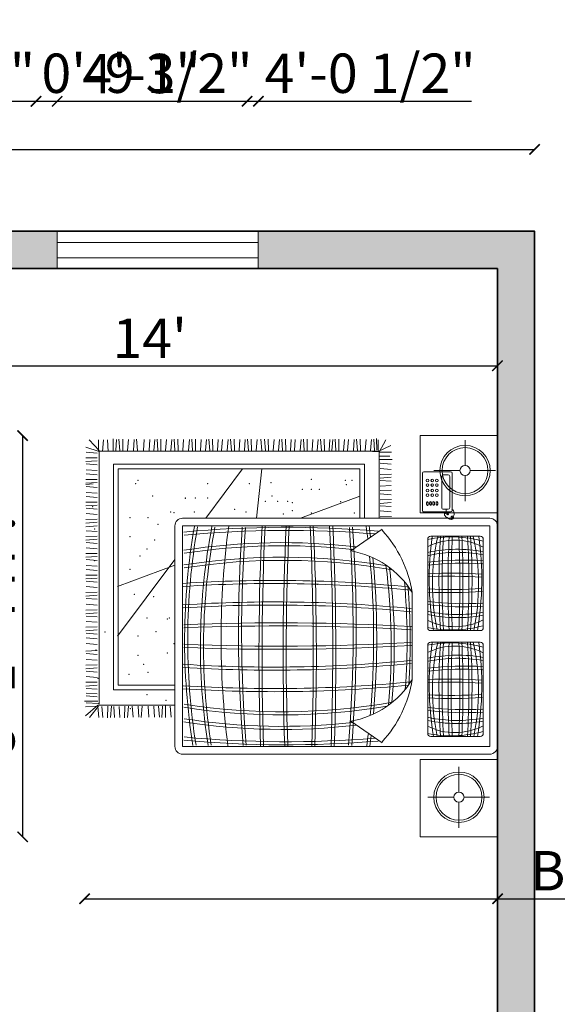
# Model space of a CAD drawing. Units: inches. Extents: x 1704 to 2334, y 1856 to 2559.
# Tile 9 of 10: x 2051 to 2180, y 2321 to 2559. Entities that reach past the tile are written whole.
import ezdxf

# ---------------------------------------------------------------- set-up
doc = ezdxf.new("R2010")
doc.units = ezdxf.units.IN
for name, color, linetype, lineweight in [('A-ANNO-DIMS', 2, 'Continuous', 18), ('A-WALL', 7, 'Continuous', 35), ('BEDS', 17, 'Continuous', 18), ('WINDOW', 6, 'Continuous', 18)]:
    doc.layers.add(name, color=color, linetype=linetype, lineweight=lineweight)
doc.layers.add('A-WALL-PATT', color=18, linetype='Continuous', lineweight=13, true_color=0x000000)
doc.styles.get("Standard").update_dxf_attribs({"font": 'arial.ttf'})
doc.dimstyles.new('ISO-25', dxfattribs={"dimtxt": 9.5, "dimasz": 2.5, "dimexe": 1.25, "dimexo": 0.625, "dimtad": 1, "dimdec": 0, "dimlunit": 4, "dimtxsty": 'Standard', "dimblk": 'ARCHTICK', "dimcen": 2.5, "dimse1": 1, "dimse2": 1, "dimclrd": 3, "dimadec": 0, "dimazin": 0, "dimtfac": 1, "dimtdec": 0, "dimtmove": 0, "dimatfit": 3, "dimfxl": 1, "dimarcsym": 0})

# ---------------------------------------------------------------- blocks, each defined once
blk = doc.blocks.new('A$C77DF40FE')
for p, q in [((0.5, 2.6723), (0, 2.6723)), ((0, 2.6723), (0, 2.1723)), ((0.226, 2.4949), (0.226, 2.6594)), ((0.5, 2.1723), (0.5, 2.6723)), ((0.5339, 0.6344), (0.5339, 2.6214)), ((0.5839, 2.6714), (2.0097, 2.6714)), ((0.5839, 2.6214), (2.0097, 2.6214)), ((0.5839, 0.6344), (0.5839, 2.6214)), ((2.0097, 2.6214), (2.0097, 0.6344)), ((2.0597, 2.6214), (2.0597, 0.6344)), ((2.0936, 2.1723), (2.0936, 2.6723)), ((2.0936, 2.6723), (2.5936, 2.6723)), ((2.3379, 2.4554), (2.3379, 2.6199)), ((2.5936, 2.6723), (2.5936, 2.1723)), ((0.6508, 2.5603), (0.6508, 2.2403)), ((1.2408, 2.5803), (0.6708, 2.5803)), ((1.2608, 2.2403), (1.2608, 2.5603)), ((1.3355, 2.5603), (1.3355, 2.2403)), ((1.9255, 2.5803), (1.3555, 2.5803)), ((1.9455, 2.2403), (1.9455, 2.5603)), ((0.0287, 2.4621), (0.1932, 2.4621)), ((0.226, 2.261), (0.226, 2.4293)), ((0.2588, 2.4621), (0.4233, 2.4621)), ((2.3051, 2.4226), (2.1406, 2.4226)), ((2.5352, 2.4226), (2.3707, 2.4226)), ((0.2338, 2.3688, 10.4), (0.2338, 2.1957, 10.4)), ((0.4828, 2.3788, 10.4), (0.2438, 2.3788, 10.4)), ((0.4656, 2.363, 10.4), (0.2638, 2.363, 10.4)), ((0.4809, 2.3823), (0.4746, 2.3757)), ((0.4873, 2.387), (0.4809, 2.3823)), ((0.4937, 2.3899), (0.4873, 2.387)), ((0.4928, 2.1957, 10.4), (0.4928, 2.3688, 10.4)), ((0.5, 2.3914), (0.4937, 2.3899)), ((0.506, 2.3917), (0.5, 2.3914)), ((0.5117, 2.391), (0.506, 2.3917)), ((0.5168, 2.3897), (0.5117, 2.391)), ((0.5212, 2.3878), (0.5168, 2.3897)), ((0.5205, 2.3816), (0.5202, 2.3804)), ((0.5202, 2.3804), (0.5202, 2.379)), ((0.5202, 2.379), (0.5206, 2.3777)), ((0.521, 2.3828), (0.5205, 2.3816)), ((0.5206, 2.3777), (0.5213, 2.3764)), ((0.5219, 2.3839), (0.521, 2.3828)), ((0.5248, 2.3858), (0.5212, 2.3878)), ((0.5213, 2.3764), (0.5224, 2.3752)), ((0.523, 2.3849), (0.5219, 2.3839)), ((0.5224, 2.3752), (0.5237, 2.374)), ((0.5244, 2.3856), (0.523, 2.3849)), ((0.5237, 2.374), (0.5252, 2.3731)), ((0.5261, 2.3861), (0.5244, 2.3856)), ((0.5277, 2.3836), (0.5248, 2.3858)), ((0.5252, 2.3731), (0.5268, 2.3723)), ((0.5279, 2.3864), (0.5261, 2.3861)), ((0.5268, 2.3723), (0.5283, 2.3719)), ((0.5298, 2.3813), (0.5277, 2.3836)), ((0.5298, 2.3864), (0.5279, 2.3864)), ((0.5283, 2.3719), (0.5297, 2.3717)), ((0.5297, 2.3717), (0.531, 2.372)), ((0.5318, 2.3861), (0.5298, 2.3864)), ((0.5313, 2.3792), (0.5298, 2.3813)), ((0.531, 2.372), (0.5319, 2.3726)), ((0.5322, 2.3771), (0.5313, 2.3792)), ((0.5338, 2.3855), (0.5318, 2.3861)), ((0.5319, 2.3726), (0.5325, 2.3738)), ((0.5326, 2.3753), (0.5322, 2.3771)), ((0.5325, 2.3738), (0.5326, 2.3753)), ((0.5356, 2.3846), (0.5338, 2.3855)), ((0.5373, 2.3832), (0.5356, 2.3846)), ((0.5356, 2.3543), (0.537, 2.3561)), ((0.537, 2.3561), (0.5383, 2.3581)), ((0.5387, 2.3815), (0.5373, 2.3832)), ((0.5383, 2.3581), (0.5394, 2.3604)), ((0.5399, 2.3794), (0.5387, 2.3815)), ((0.5394, 2.3604), (0.5403, 2.3629)), ((0.5407, 2.377), (0.5399, 2.3794)), ((0.5403, 2.3629), (0.5409, 2.3657)), ((0.5412, 2.3743), (0.5407, 2.377)), ((0.5409, 2.3657), (0.5413, 2.3686)), ((0.5414, 2.3715), (0.5412, 2.3743)), ((0.5413, 2.3686), (0.5414, 2.3715)), ((2.3379, 2.2215), (2.3379, 2.3898)), ((0.2538, 2.353, 10.4), (0.2538, 2.3215, 10.4)), ((0.2638, 2.3115, 10.4), (0.4656, 2.3115, 10.4)), ((0.4756, 2.3215, 10.4), (0.4756, 2.353, 10.4)), ((0.4767, 2.3409), (0.4876, 2.34)), ((0.4876, 2.34), (0.4961, 2.3402)), ((0.4961, 2.3402), (0.5023, 2.3413)), ((0.502, 2.3463), (0.5017, 2.3431)), ((0.5017, 2.3431), (0.5018, 2.3398)), ((0.5018, 2.3398), (0.5023, 2.3365)), ((0.5026, 2.3491), (0.502, 2.3463)), ((0.5023, 2.3413), (0.5067, 2.3431)), ((0.5023, 2.3365), (0.5031, 2.3334)), ((0.5035, 2.3514), (0.5026, 2.3491)), ((0.5031, 2.3334), (0.5043, 2.3309)), ((0.5047, 2.3531), (0.5035, 2.3514)), ((0.5043, 2.3309), (0.506, 2.329)), ((0.5059, 2.3542), (0.5047, 2.3531)), ((0.5073, 2.3548), (0.5059, 2.3542)), ((0.506, 2.329), (0.5081, 2.328)), ((0.5067, 2.3431), (0.5095, 2.3452)), ((0.5086, 2.3549), (0.5073, 2.3548)), ((0.5081, 2.328), (0.5106, 2.328)), ((0.5097, 2.3544), (0.5086, 2.3549)), ((0.5095, 2.3452), (0.511, 2.3475)), ((0.5107, 2.3534), (0.5097, 2.3544)), ((0.5106, 2.328), (0.5134, 2.3288)), ((0.5113, 2.3518), (0.5107, 2.3534)), ((0.511, 2.3475), (0.5115, 2.3498)), ((0.5115, 2.3498), (0.5113, 2.3518)), ((0.5134, 2.3288), (0.5163, 2.3304)), ((0.5163, 2.3304), (0.5193, 2.3325)), ((0.5193, 2.3325), (0.5222, 2.3349)), ((0.5222, 2.3349), (0.5249, 2.3374)), ((0.5249, 2.3374), (0.5271, 2.3398)), ((0.5271, 2.3398), (0.5288, 2.3419)), ((0.5288, 2.3419), (0.5299, 2.3436)), ((0.5299, 2.3436), (0.5305, 2.3449)), ((0.53, 2.3482), (0.5302, 2.3488)), ((0.5301, 2.3477), (0.53, 2.3482)), ((0.5303, 2.3472), (0.5301, 2.3477)), ((0.5302, 2.3488), (0.5308, 2.3495)), ((0.5306, 2.3466), (0.5303, 2.3472)), ((0.5305, 2.3449), (0.5307, 2.3459)), ((0.5307, 2.3459), (0.5306, 2.3466)), ((0.5308, 2.3495), (0.5317, 2.3504)), ((0.5317, 2.3504), (0.5329, 2.3515)), ((0.5329, 2.3515), (0.5342, 2.3528)), ((0.5342, 2.3528), (0.5356, 2.3543)), ((0, 2.1723), (0.5, 2.1723)), ((0.2438, 2.1857, 10.4), (0.4828, 2.1857, 10.4)), ((0.6708, 2.2203), (1.2408, 2.2203)), ((1.3555, 2.2203), (1.9255, 2.2203)), ((2.5936, 2.1723), (2.0936, 2.1723)), ((1.5773, 2.1205), (1.0147, 2.1205)), ((0.0644, 1.9807), (0.1019, 1.9003)), ((0.1072, 1.986), (0.1072, 1.911)), ((0.134, 1.9753), (0.134, 1.9057)), ((0.1554, 1.9914), (0.1554, 1.911)), ((0.1792, 1.9138), (0.1849, 1.9847)), ((0.2134, 1.9138), (0.219, 1.9847)), ((0.251, 1.9118), (0.2494, 1.9865)), ((0.2748, 1.9118), (0.2691, 1.9849)), ((0.2899, 1.9138), (0.2956, 1.9847)), ((0.3277, 1.9118), (0.3219, 1.9849)), ((0.3539, 1.9118), (0.3522, 1.9865)), ((0.3766, 1.9138), (0.3822, 1.9847)), ((0.4142, 1.9118), (0.4126, 1.9865)), ((0.438, 1.9118), (0.4323, 1.9849)), ((0.4531, 1.9138), (0.4588, 1.9847)), ((0.4873, 1.9138), (0.493, 1.9847)), ((0.5249, 1.9118), (0.5233, 1.9865)), ((0.1072, 1.9057), (0.0269, 1.9485)), ((0.6051, 1.925), (0.7457, 1.7234)), ((1.9869, 1.925), (1.8463, 1.7234)), ((0.0195, 1.8887), (0.0942, 1.8903)), ((0.0227, 1.8712), (0.0957, 1.8769)), ((0.0247, 1.8561), (0.0955, 1.8504)), ((0.1019, 1.9003), (0.0269, 1.9003)), ((0.1002, 1.8885), (0.1002, 0.0935)), ((0.3112, 1.9057), (0.1019, 1.9057)), ((0.1019, 1.9057), (0.1019, 1.8628)), ((0.5301, 1.9057), (0.3112, 1.9057)), ((0.0227, 1.7843), (0.0974, 1.786)), ((0.0247, 1.8219), (0.0955, 1.8163)), ((0.3112, 1.8116), (0.1852, 1.8116)), ((0.1852, 1.8116), (0.1852, 0.187)), ((0.5339, 1.8116), (0.3112, 1.8116)), ((0.0227, 1.7605), (0.0957, 1.7662)), ((0.0247, 1.7454), (0.0955, 1.7397)), ((0.3112, 1.7816), (0.2152, 1.7816)), ((0.2152, 1.7816), (0.2152, 0.217)), ((0.5339, 1.7816), (0.3112, 1.7816)), ((0.3909, 1.7821), (0.5339, 1.398)), ((0.0247, 1.708), (0.0955, 1.7023)), ((0.0247, 1.6819), (0.0955, 1.6762)), ((0.0227, 1.6443), (0.0974, 1.6459)), ((0.0227, 1.6205), (0.0957, 1.6262)), ((0.0247, 1.6054), (0.0955, 1.5997)), ((0.0227, 1.5505), (0.0974, 1.5521)), ((0.0227, 1.5266), (0.0957, 1.5324)), ((0.0247, 1.5881), (0.0955, 1.5824)), ((0.0247, 1.5116), (0.0955, 1.5059)), ((0.0247, 1.4774), (0.0955, 1.4717)), ((0.0227, 1.4397), (0.0974, 1.4414)), ((0.0227, 1.4159), (0.0957, 1.4217)), ((0.0247, 1.4008), (0.0955, 1.3952)), ((0.0247, 1.3634), (0.0955, 1.3577)), ((0.0247, 1.3374), (0.0955, 1.3317)), ((0.0227, 1.2997), (0.0974, 1.3014)), ((0.0227, 1.2759), (0.0957, 1.2816)), ((0.0247, 1.2608), (0.0955, 1.2551)), ((0.0247, 1.2266), (0.0955, 1.221)), ((0.0227, 1.189), (0.0974, 1.1906)), ((0.0227, 1.1652), (0.0957, 1.1709)), ((0.0227, 1.1414), (0.0957, 1.1471)), ((0.5339, 1.1132), (0.2152, 1.1479)), ((0.0247, 1.1163), (0.0955, 1.1106)), ((0.0227, 1.0786), (0.0974, 1.0803)), ((0.0227, 1.0548), (0.0957, 1.0606)), ((0.0247, 1.0397), (0.0955, 1.0341)), ((0.5339, 0.7837), (0.2152, 1.0221)), ((0.0227, 0.9679), (0.0974, 0.9696)), ((0.0247, 1.0055), (0.0955, 0.9999)), ((0.0227, 0.9441), (0.0957, 0.9498)), ((0.0247, 0.929), (0.0955, 0.9233)), ((0.0247, 0.8916), (0.0955, 0.8859)), ((0.0227, 0.8279), (0.0974, 0.8295)), ((0.0247, 0.8655), (0.0955, 0.8599)), ((0.0227, 0.8041), (0.0957, 0.8098)), ((0.0247, 0.789), (0.0955, 0.7833)), ((0.0227, 0.7172), (0.0974, 0.7188)), ((0.0247, 0.7548), (0.0955, 0.7491)), ((0.0227, 0.6933), (0.0957, 0.6991)), ((0.0247, 0.6783), (0.0955, 0.6726)), ((0.0247, 0.6408), (0.0955, 0.6352)), ((0.0227, 0.6032), (0.0974, 0.6048)), ((0.0227, 0.5794), (0.0957, 0.5851)), ((2.0097, 0.6344), (0.5839, 0.6344)), ((2.0097, 0.5844), (0.5839, 0.5844)), ((1.2963, 0.2134), (0.8003, 0.5844)), ((0.8369, 0.5844), (0.975, 0.2134)), ((1.6139, 0.217), (1.6139, 0.5844)), ((1.6439, 0.187), (1.6439, 0.5844)), ((1.7439, 0.087), (1.7439, 0.5844)), ((0.0247, 0.5643), (0.0955, 0.5586)), ((0.0247, 0.5301), (0.0955, 0.5244)), ((1.8218, 0.5229), (1.7471, 0.5245)), ((1.8197, 0.5605), (1.7489, 0.5548)), ((0.0227, 0.4925), (0.0974, 0.4941)), ((0.0227, 0.4687), (0.0957, 0.4744)), ((0.0247, 0.4536), (0.0955, 0.4479)), ((1.8218, 0.499), (1.7487, 0.5048)), ((1.8197, 0.4839), (1.7489, 0.4783)), ((1.8197, 0.453), (1.7489, 0.4474)), ((0.0247, 0.4227), (0.0955, 0.417)), ((0.0247, 0.3864), (0.0955, 0.3807)), ((1.8197, 0.4168), (1.7489, 0.4111)), ((0.0227, 0.3367), (0.0957, 0.3424)), ((0.0247, 0.3216), (0.0955, 0.3159)), ((1.8218, 0.3671), (1.7487, 0.3728)), ((1.8197, 0.352), (1.7489, 0.3463)), ((0.0247, 0.2842), (0.0955, 0.2785)), ((1.8197, 0.3146), (1.7489, 0.3089)), ((1.7492, 0.2844), (1.8223, 0.2787)), ((1.7492, 0.2606), (1.824, 0.2589)), ((0.0227, 0.2465), (0.0974, 0.2482)), ((0.0227, 0.2227), (0.0957, 0.2285)), ((0.0247, 0.2076), (0.0955, 0.202)), ((0.2152, 0.217), (0.3112, 0.217)), ((0.3112, 0.217), (1.6139, 0.217)), ((1.7513, 0.223), (1.8221, 0.2286)), ((1.7513, 0.1888), (1.8221, 0.1944)), ((0.1019, 0.1857), (0.0216, 0.1857)), ((0.1019, 0.1535), (0.0269, 0.1482)), ((0.1852, 0.187), (0.3112, 0.187)), ((0.3112, 0.187), (1.6439, 0.187)), ((1.7492, 0.1737), (1.8223, 0.1679)), ((1.7492, 0.1499), (1.824, 0.1482)), ((0.1019, 0.116), (0.0269, 0.1214)), ((0.0965, 0.0946), (0.0269, 0.0303)), ((0.1019, 0.0892), (0.0269, 0.0892)), ((0.1019, 0.0946), (0.0751, 0.0089)), ((0.1002, 0.0935), (0.3112, 0.0935)), ((0.107, 0.0096), (0.1126, 0.0804)), ((0.1446, 0.0075), (0.1429, 0.0823)), ((0.1684, 0.0075), (0.1627, 0.0806)), ((0.1835, 0.0096), (0.1892, 0.0804)), ((0.2209, 0.0096), (0.2266, 0.0804)), ((0.247, 0.0096), (0.2527, 0.0804)), ((0.2846, 0.0075), (0.283, 0.0823)), ((0.3084, 0.0075), (0.3027, 0.0806)), ((0.3112, 0.0935), (1.0155, 0.0935)), ((0.3301, 0.0096), (0.3358, 0.0804)), ((0.3676, 0.0096), (0.3732, 0.0804)), ((0.3936, 0.0096), (0.3993, 0.0804)), ((0.4313, 0.0075), (0.4296, 0.0823)), ((0.4551, 0.0075), (0.4493, 0.0806)), ((0.4702, 0.0096), (0.4758, 0.0804)), ((0.5043, 0.0096), (0.51, 0.0804)), ((0.542, 0.0075), (0.5403, 0.0823)), ((0.5658, 0.0075), (0.56, 0.0806)), ((0.5896, 0.0075), (0.5838, 0.0806)), ((0.6147, 0.0096), (0.6204, 0.0804)), ((0.6523, 0.0075), (0.6507, 0.0823)), ((0.6762, 0.0075), (0.6704, 0.0806)), ((0.6912, 0.0096), (0.6969, 0.0804)), ((0.7254, 0.0096), (0.7311, 0.0804)), ((0.7631, 0.0075), (0.7614, 0.0823)), ((0.7869, 0.0075), (0.7811, 0.0806)), ((0.802, 0.0096), (0.8076, 0.0804)), ((0.8394, 0.0096), (0.8451, 0.0804)), ((0.8654, 0.0096), (0.8711, 0.0804)), ((0.9031, 0.0075), (0.9014, 0.0823)), ((0.9269, 0.0075), (0.9212, 0.0806)), ((0.942, 0.0096), (0.9477, 0.0804)), ((0.9762, 0.0096), (0.9818, 0.0804)), ((1.0138, 0.0075), (1.0122, 0.0823)), ((1.0155, 0.0935), (1.7355, 0.0935)), ((1.0376, 0.0075), (1.0319, 0.0806)), ((1.0527, 0.0096), (1.0584, 0.0804)), ((1.0901, 0.0096), (1.0958, 0.0804)), ((1.1278, 0.0075), (1.1261, 0.0823)), ((1.1516, 0.0075), (1.1459, 0.0806)), ((1.1667, 0.0096), (1.1724, 0.0804)), ((1.2009, 0.0096), (1.2065, 0.0804)), ((1.2385, 0.0075), (1.2368, 0.0823)), ((1.2623, 0.0075), (1.2566, 0.0806)), ((1.2774, 0.0096), (1.2831, 0.0804)), ((1.3083, 0.0096), (1.314, 0.0804)), ((1.3446, 0.0096), (1.3503, 0.0804)), ((1.3943, 0.0075), (1.3885, 0.0806)), ((1.4094, 0.0096), (1.415, 0.0804)), ((1.4468, 0.0096), (1.4525, 0.0804)), ((1.4844, 0.0075), (1.4828, 0.0823)), ((1.5083, 0.0075), (1.5025, 0.0806)), ((1.5233, 0.0096), (1.529, 0.0804)), ((1.5575, 0.0096), (1.5632, 0.0804)), ((1.5951, 0.0075), (1.5935, 0.0823)), ((1.619, 0.0075), (1.6132, 0.0806)), ((1.6341, 0.0096), (1.6397, 0.0804)), ((1.665, 0.0096), (1.6706, 0.0804)), ((1.6831, 0.0096), (1.6888, 0.0804)), ((1.7162, 0.0857), (1.7162, 0)), ((1.7323, 0.0911), (1.7269, 0.0107)), ((1.743, 0.0857), (1.8126, 0.0054)), ((1.7483, 0.0911), (1.8233, 0.0322)), ((1.7483, 0.0857), (1.7537, 0.0054)), ((1.7513, 0.1122), (1.8221, 0.1179)), ((1.7513, 0.0858), (1.8221, 0.0915)), ((0.3151, 0.0075), (0.3112, 0.0565))]:
    blk.add_line(p, q)
for centre, radius in [((0.226, 2.4621), 0.1629), ((0.226, 2.4621), 0.1484), ((2.3379, 2.4226), 0.1629), ((2.3379, 2.4226), 0.1484), ((0.226, 2.4621), 0.0328), ((2.3379, 2.4226), 0.0328), ((0.2896, 2.2801, 10.4), 0.00858), ((0.2896, 2.25, 10.4), 0.00858), ((0.3196, 2.2801, 10.4), 0.00858), ((0.3196, 2.25, 10.4), 0.00858), ((0.3554, 2.2801, 10.4), 0.00858), ((0.3554, 2.25, 10.4), 0.00858), ((0.3855, 2.2801, 10.4), 0.00858), ((0.3855, 2.25, 10.4), 0.00858), ((0.2896, 2.2186, 10.4), 0.00858), ((0.3196, 2.2186, 10.4), 0.00858), ((0.3554, 2.2186, 10.4), 0.00858), ((0.3855, 2.2186, 10.4), 0.00858)]:
    blk.add_circle(centre, radius)
for centre, radius, start, end in [((0.5839, 2.6214), 0.05, 90, 180), ((2.0097, 2.6214), 0.05, 0, 90), ((0.6708, 2.5603), 0.02, 90, 180), ((0.9635, 1.1066), 1.4427, 78.1527, 102.49062), ((0.9287, 0.5819), 1.9884, 80.42006, 97.96719), ((1.4247, 2.3742), 0.7696, 164.61122, 191.56793), ((1.0701, 2.3966), 0.3942, 152.53654, 206.92003), ((1.6628, 2.4129), 0.928, 169.60866, 191.89899), ((1.6628, 2.4129), 0.908, 169.60866, 191.89899), ((2.7571, 2.4533), 1.9523, 176.39469, 186.81952), ((2.7571, 2.4533), 1.9323, 176.39469, 186.81952), ((3.9259, 2.3685), 3.0367, 176.14325, 182.77497), ((3.9259, 2.3685), 3.0167, 176.14325, 182.77497), ((-2.0216, 2.3685), 3.0167, 357.22503, 3.85675), ((-2.0216, 2.3685), 3.0367, 357.22503, 3.85675), ((-0.8455, 2.4533), 1.9323, 353.18048, 3.60531), ((-0.8455, 2.4533), 1.9523, 353.18048, 3.60531), ((0.2489, 2.4129), 0.908, 348.10101, 10.39134), ((0.2489, 2.4129), 0.928, 348.10101, 10.39134), ((0.8416, 2.3966), 0.3942, 333.07997, 27.46346), ((0.4869, 2.3742), 0.7696, 348.43207, 15.38878), ((1.2408, 2.5603), 0.02, 0, 90), ((1.3555, 2.5603), 0.02, 90, 180), ((1.6482, 1.1066), 1.4427, 78.1527, 102.49062), ((1.6135, 0.5819), 1.9884, 80.42006, 97.96719), ((2.1094, 2.3742), 0.7696, 164.61122, 191.56793), ((1.7548, 2.3966), 0.3942, 152.53654, 206.92003), ((2.3475, 2.4129), 0.928, 169.60866, 191.89899), ((2.3475, 2.4129), 0.908, 169.60866, 191.89899), ((3.4419, 2.4533), 1.9523, 176.39469, 186.81952), ((3.4419, 2.4533), 1.9323, 176.39469, 186.81952), ((4.6106, 2.3685), 3.0367, 176.14325, 182.77497), ((4.6106, 2.3685), 3.0167, 176.14325, 182.77497), ((-1.3369, 2.3685), 3.0167, 357.22503, 3.85675), ((-1.3369, 2.3685), 3.0367, 357.22503, 3.85675), ((-0.1608, 2.4533), 1.9323, 353.18048, 3.60531), ((-0.1608, 2.4533), 1.9523, 353.18048, 3.60531), ((0.9336, 2.4129), 0.908, 348.10101, 10.39134), ((0.9336, 2.4129), 0.928, 348.10101, 10.39134), ((1.5263, 2.3966), 0.3942, 333.07997, 27.46346), ((1.1716, 2.3742), 0.7696, 348.43207, 15.38878), ((1.9255, 2.5603), 0.02, 0, 90), ((0.9445, -2.3575), 4.8647, 86.26705, 93.45634), ((0.9445, -2.3575), 4.8447, 86.26705, 93.45634), ((1.6292, -2.3575), 4.8647, 86.26705, 93.45634), ((1.6292, -2.3575), 4.8447, 86.26705, 93.45634), ((0.9561, -3.928), 6.3765, 87.24779, 92.75221), ((0.9561, -3.928), 6.3565, 87.24779, 92.75221), ((1.6408, -3.928), 6.3765, 87.24779, 92.75221), ((1.6408, -3.928), 6.3565, 87.24779, 92.75221), ((0.2438, 2.3688, 10.4), 0.01, 90, 180), ((0.2638, 2.353, 10.4), 0.01, 90, 180), ((0.4656, 2.353, 10.4), 0.01, 0, 90), ((0.4828, 2.3688, 10.4), 0.01, 0, 90), ((0.9561, 8.7285), 6.3765, 267.24779, 272.75221), ((0.9561, 8.7285), 6.3565, 267.24779, 272.75221), ((1.6408, 8.7285), 6.3765, 267.24779, 272.75221), ((1.6408, 8.7285), 6.3565, 267.24779, 272.75221), ((0.2638, 2.3215, 10.4), 0.01, 180, 270), ((0.4656, 2.3215, 10.4), 0.01, 270, 0), ((0.9445, 7.158), 4.8647, 266.54366, 273.73295), ((0.9445, 7.158), 4.8447, 266.54366, 273.73295), ((1.6292, 7.158), 4.8647, 266.54366, 273.73295), ((1.6292, 7.158), 4.8447, 266.54366, 273.73295), ((0.43, 2.2801, 10.4), 0.00304, 140.36073, 180), ((0.43, 2.2801, 10.4), 0.00304, 180, 219.63927), ((0.43, 2.2586, 10.4), 0.00304, 140.36073, 180), ((0.43, 2.2586, 10.4), 0.00304, 180, 219.63927), ((0.43, 2.2386, 10.4), 0.00304, 140.36073, 180), ((0.43, 2.2386, 10.4), 0.00304, 180, 219.63927), ((0.434, 2.2768, 10.4), 0.00822, 116.56505, 140.36073), ((0.434, 2.2834, 10.4), 0.00822, 219.63927, 243.43495), ((0.434, 2.2553, 10.4), 0.00822, 116.56505, 140.36073), ((0.434, 2.2619, 10.4), 0.00822, 219.63927, 243.43495), ((0.434, 2.2353, 10.4), 0.00822, 116.56505, 140.36073), ((0.434, 2.2419, 10.4), 0.00822, 219.63927, 243.43495), ((0.4367, 2.2714, 10.4), 0.0142, 101.70092, 116.56505), ((0.4367, 2.2887, 10.4), 0.0142, 243.43495, 258.29908), ((0.4367, 2.25, 10.4), 0.0142, 101.70092, 116.56505), ((0.4367, 2.2673, 10.4), 0.0142, 243.43495, 258.29908), ((0.4367, 2.23, 10.4), 0.0142, 101.70092, 116.56505), ((0.4367, 2.2472, 10.4), 0.0142, 243.43495, 258.29908), ((0.4384, 2.263, 10.4), 0.0228, 90, 101.70092), ((0.4384, 2.2972, 10.4), 0.0228, 258.29908, 270), ((0.4384, 2.2415, 10.4), 0.0228, 90, 101.70092), ((0.4384, 2.2757, 10.4), 0.0228, 258.29908, 270), ((0.4384, 2.2215, 10.4), 0.0228, 90, 101.70092), ((0.4384, 2.2557, 10.4), 0.0228, 258.29908, 270), ((0.4384, 2.263, 10.4), 0.0228, 78.29908, 90), ((0.4384, 2.2972, 10.4), 0.0228, 270, 281.70092), ((0.4384, 2.2415, 10.4), 0.0228, 78.29908, 90), ((0.4384, 2.2757, 10.4), 0.0228, 270, 281.70092), ((0.4384, 2.2215, 10.4), 0.0228, 78.29908, 90), ((0.4384, 2.2557, 10.4), 0.0228, 270, 281.70092), ((0.4402, 2.2714, 10.4), 0.0142, 63.43495, 78.29908), ((0.4402, 2.2887, 10.4), 0.0142, 281.70092, 296.56505), ((0.4402, 2.25, 10.4), 0.0142, 63.43495, 78.29908), ((0.4402, 2.2673, 10.4), 0.0142, 281.70092, 296.56505), ((0.4402, 2.23, 10.4), 0.0142, 63.43495, 78.29908), ((0.4402, 2.2472, 10.4), 0.0142, 281.70092, 296.56505), ((0.4428, 2.2768, 10.4), 0.00822, 39.63927, 63.43495), ((0.4428, 2.2834, 10.4), 0.00822, 296.56505, 320.36073), ((0.4428, 2.2553, 10.4), 0.00822, 39.63927, 63.43495), ((0.4428, 2.2619, 10.4), 0.00822, 296.56505, 320.36073), ((0.4428, 2.2353, 10.4), 0.00822, 39.63927, 63.43495), ((0.4428, 2.2419, 10.4), 0.00822, 296.56505, 320.36073), ((0.4468, 2.2801, 10.4), 0.00304, 0, 39.63927), ((0.4468, 2.2801, 10.4), 0.00304, 320.36073, 0), ((0.4468, 2.2586, 10.4), 0.00304, 0, 39.63927), ((0.4468, 2.2586, 10.4), 0.00304, 320.36073, 0), ((0.4468, 2.2386, 10.4), 0.00304, 0, 39.63927), ((0.4468, 2.2386, 10.4), 0.00304, 320.36073, 0), ((0.6708, 2.2403), 0.02, 180, 270), ((0.9635, 3.6939), 1.4427, 257.50938, 281.8473), ((0.9287, 4.2186), 1.9884, 262.03281, 279.57994), ((1.2408, 2.2403), 0.02, 270, 0), ((1.3555, 2.2403), 0.02, 180, 270), ((1.6482, 3.6939), 1.4427, 257.50938, 281.8473), ((1.6135, 4.2186), 1.9884, 262.03281, 279.57994), ((1.9255, 2.2403), 0.02, 270, 0), ((0.2438, 2.1957, 10.4), 0.01, 180, 270), ((0.4314, 2.2186, 10.4), 0.00304, 140.36073, 180), ((0.4314, 2.2186, 10.4), 0.00304, 180, 219.63927), ((0.4354, 2.2153, 10.4), 0.00822, 116.56505, 140.36073), ((0.4354, 2.2219, 10.4), 0.00822, 219.63927, 243.43495), ((0.4381, 2.2099, 10.4), 0.0142, 101.70092, 116.56505), ((0.4381, 2.2272, 10.4), 0.0142, 243.43495, 258.29908), ((0.4398, 2.2015, 10.4), 0.0228, 90, 101.70092), ((0.4398, 2.2357, 10.4), 0.0228, 258.29908, 270), ((0.4398, 2.2015, 10.4), 0.0228, 78.29908, 90), ((0.4398, 2.2357, 10.4), 0.0228, 270, 281.70092), ((0.4416, 2.2099, 10.4), 0.0142, 63.43495, 78.29908), ((0.4416, 2.2272, 10.4), 0.0142, 281.70092, 296.56505), ((0.4443, 2.2153, 10.4), 0.00822, 39.63927, 63.43495), ((0.4443, 2.2219, 10.4), 0.00822, 296.56505, 320.36073), ((0.4483, 2.2186, 10.4), 0.00304, 0, 39.63927), ((0.4483, 2.2186, 10.4), 0.00304, 320.36073, 0), ((0.4828, 2.1957, 10.4), 0.01, 270, 0), ((1.1396, 1.3485), 0.782, 99.19081, 132.51156), ((1.3217, 1.6229), 0.5847, 121.66764, 170.10648), ((10.1174, 1.2237), 9.161, 174.43278, 183.67204), ((1.3248, -2.1722), 4.2793, 86.15317, 94.70908), ((10.2564, 1.2237), 9.181, 174.43278, 183.67204), ((10.2564, 1.2237), 9.161, 174.43278, 183.67204), ((16.3019, 1.253), 15.0916, 176.72768, 182.32074), ((16.3019, 1.253), 15.0716, 176.72768, 182.32074), ((-13.7099, 1.253), 15.0716, 357.67926, 3.27232), ((-13.7099, 1.253), 15.0916, 357.67926, 3.27232), ((-7.6644, 1.2237), 9.161, 356.32796, 5.56722), ((-7.6644, 1.2237), 9.181, 356.32796, 5.56722), ((1.2703, 1.6229), 0.5847, 9.89352, 58.33236), ((1.4523, 1.3485), 0.782, 47.48844, 80.80919), ((-7.5254, 1.2237), 9.161, 356.32796, 5.55658), ((10.1174, 1.2237), 9.181, 174.54912, 183.67204), ((1.3248, -2.1722), 4.2593, 85.74731, 95.1159), ((-7.5254, 1.2237), 9.181, 356.32796, 5.45088), ((4.947, 1.2796), 4.1406, 170.09388, 188.81788), ((1.3657, -2.1044), 4.0888, 84.7053, 97.42828), ((1.3657, -2.1044), 4.1088, 84.96186, 97.17068), ((-2.355, 1.2796), 4.1406, 351.18212, 9.90612), ((4.947, 1.2796), 4.1606, 170.62723, 188.81788), ((-2.355, 1.2796), 4.1606, 351.18212, 9.37277), ((1.3142, -3.5764), 5.4671, 96.90782, 97.69237), ((7.8077, 1.3061), 7.2149, 175.27403, 185.28261), ((7.8077, 1.3061), 7.1949, 175.41729, 185.28261), ((1.3142, -3.5764), 5.4471, 84.77918, 95.62141), ((1.3142, -3.5764), 5.4671, 84.89528, 95.50522), ((1.3142, -3.5764), 5.4671, 82.70251, 83.44735), ((-5.2157, 1.3061), 7.1949, 354.71739, 4.58271), ((-5.2157, 1.3061), 7.2149, 354.71739, 4.72597), ((1.3142, -3.5764), 5.4471, 96.79597, 97.69237), ((1.3142, -3.5764), 5.4471, 82.70251, 83.56088), ((1.2659, -7.4764), 9.2344, 85.41732, 94.18368), ((1.2659, -7.4764), 9.2144, 85.41732, 94.18368), ((4.8527, 1.2796), 4.1606, 173.36767, 188.81788), ((4.8527, 1.2796), 4.1406, 173.68117, 188.81788), ((-2.2608, 1.2796), 4.1406, 351.18212, 6.31883), ((-2.2608, 1.2796), 4.1606, 351.18212, 6.63233), ((1.4138, -15.5462), 17.172, 88.01473, 92.775), ((1.4138, -15.5462), 17.152, 88.01473, 92.775), ((1.4138, -15.6721), 17.172, 88.01473, 92.775), ((1.4138, -15.6721), 17.152, 88.01473, 92.775), ((1.4138, 18.4566), 17.172, 267.225, 271.98527), ((1.4138, 18.4566), 17.152, 267.225, 271.98527), ((1.4138, 18.3004), 17.172, 267.225, 271.98527), ((1.4138, 18.3004), 17.152, 267.225, 271.98527), ((1.2659, 10.2305), 9.2344, 265.81632, 274.58268), ((1.2659, 10.2305), 9.2144, 265.81632, 274.58268), ((1.3142, 6.3306), 5.4471, 262.30763, 277.29749), ((1.3657, 4.8586), 4.0888, 259.07937, 278.93274), ((1.3657, 4.8586), 4.1088, 259.07937, 278.93274), ((1.3248, 4.9264), 4.2793, 260.07608, 279.1287), ((1.3248, 4.9264), 4.2593, 260.07608, 279.1287), ((0.5839, 0.6344), 0.05, 180, 270), ((2.0097, 0.6344), 0.05, 270, 0)]:
    blk.add_arc(centre, radius, start, end)
for p in [(0.2895, 1.7311), (0.5004, 1.7457), (0.2895, 1.6873), (0.3179, 1.6946), (0.4274, 1.6581), (0.2822, 1.4684), (0.3471, 1.5195), (0.3471, 1.4684), (0.5004, 1.4684), (0.9622, 1.5058), (0.3471, 1.41), (0.4326, 1.3443), (0.4858, 1.3444), (0.4253, 1.3151), (0.5077, 1.286), (0.3909, 1.213), (0.4253, 1.2495), (0.3041, 1.2057), (0.4253, 1.1692), (0.3106, 1.0671), (0.4931, 1.0452), (0.4765, 0.9722), (0.3114, 0.7971), (0.4034, 0.7971), (0.4034, 0.7169), (0.4931, 0.7096), (0.4034, 0.6512), (0.4055, 0.6512), (0.4984, 0.5782), (1.3453, 0.5782), (0.4931, 0.5564), (1.1794, 0.5491), (1.1867, 0.5345), (1.4058, 0.5345), (1.7124, 0.5272), (0.5734, 0.4761), (0.6757, 0.4542), (1.0407, 0.4469), (1.2671, 0.4615), (0.3909, 0.4396), (0.5296, 0.4104), (0.7341, 0.4032), (1.1794, 0.4032), (1.5299, 0.4104), (1.6759, 0.4032), (0.2895, 0.3448), (0.3114, 0.3302), (0.7779, 0.3594), (1.0261, 0.3229), (1.2963, 0.3448), (1.4204, 0.3448), (1.4788, 0.3813), (0.5296, 0.2937), (0.6538, 0.2937), (0.8655, 0.2937), (1.5445, 0.2864), (1.7652, 0.2958), (1.2693, 0.1315), (0.6049, 0.0659), (0.8093, 0.0659), (1.3861, 0.0732), (1.5686, 0.0878), (0.4588, 0.0513)]:
    blk.add_point(p)
blk = doc.blocks.new('_ArchTick')
at = {"color": 0, "linetype": 'ByBlock', "const_width": 0.15}
blk.add_lwpolyline([(-0.5, -0.5), (0.5, 0.5)], dxfattribs=at)
blk = doc.blocks.new('*D14')
at = {"layer": 'A-ANNO-DIMS', "color": 0, "lineweight": -2, "transparency": 16777216}
blk.add_line((1998.01, 2475.56), (2166.01, 2475.56), dxfattribs=at)
at = {"layer": 'Defpoints', "color": 0, "transparency": 16777216}
for p in [(2166.01, 2475.56), (1998.01, 2469.33), (2166.01, 2469.33)]:
    blk.add_point(p, dxfattribs=at)
at = {"layer": 'A-ANNO-DIMS', "color": 0, "lineweight": -2, "transparency": 16777216, "xscale": 2.5, "yscale": 2.5, "zscale": 2.5, "rotation": 180}
blk.add_blockref('_ArchTick', (1998.01, 2475.56), dxfattribs=at)
at = {"layer": 'A-ANNO-DIMS', "color": 0, "lineweight": -2, "transparency": 16777216, "xscale": 2.5, "yscale": 2.5, "zscale": 2.5}
blk.add_blockref('_ArchTick', (2166.01, 2475.56), dxfattribs=at)
at = {"layer": 'A-ANNO-DIMS', "color": 0, "transparency": 16777216, "insert": (2082.01, 2480.96), "char_height": 9.5, "attachment_point": 5}
blk.add_mtext("14'", dxfattribs=at)
blk = doc.blocks.new('*D22')
at = {"layer": 'A-ANNO-DIMS', "color": 0, "lineweight": -2, "transparency": 16777216}
blk.add_line((1755.01, 2527.77), (2175.01, 2527.77), dxfattribs=at)
at = {"layer": 'Defpoints', "color": 0, "transparency": 16777216}
for p in [(2175.01, 2527.77), (1755.01, 2508.04), (2175.01, 2508.04)]:
    blk.add_point(p, dxfattribs=at)
at = {"layer": 'A-ANNO-DIMS', "color": 0, "lineweight": -2, "transparency": 16777216, "xscale": 2.5, "yscale": 2.5, "zscale": 2.5, "rotation": 180}
blk.add_blockref('_ArchTick', (1755.01, 2527.77), dxfattribs=at)
at = {"layer": 'A-ANNO-DIMS', "color": 0, "lineweight": -2, "transparency": 16777216, "xscale": 2.5, "yscale": 2.5, "zscale": 2.5}
blk.add_blockref('_ArchTick', (2175.01, 2527.77), dxfattribs=at)
at = {"layer": 'A-ANNO-DIMS', "color": 0, "transparency": 16777216, "insert": (1965.01, 2533.25), "char_height": 9.5, "attachment_point": 5}
blk.add_mtext("35'", dxfattribs=at)
blk = doc.blocks.new('*D24')
at = {"layer": 'A-ANNO-DIMS', "color": 3, "lineweight": -2, "transparency": 16777216}
for p, q in [((2066.27, 2346.88), (2166.04, 2346.88)), ((2166.04, 2346.88), (2334.22, 2346.88))]:
    blk.add_line(p, q, dxfattribs=at)
at = {"layer": 'Defpoints', "color": 0, "transparency": 16777216}
for p in [(2066.27, 2361.85), (2166.04, 2361.85), (2166.04, 2346.88)]:
    blk.add_point(p, dxfattribs=at)
at = {"layer": 'A-ANNO-DIMS', "color": 3, "lineweight": -2, "transparency": 16777216, "xscale": 2.5, "yscale": 2.5, "zscale": 2.5, "rotation": 180}
blk.add_blockref('_ArchTick', (2066.27, 2346.88), dxfattribs=at)
at = {"layer": 'A-ANNO-DIMS', "color": 3, "lineweight": -2, "transparency": 16777216, "xscale": 2.5, "yscale": 2.5, "zscale": 2.5}
blk.add_blockref('_ArchTick', (2166.04, 2346.88), dxfattribs=at)
at = {"layer": 'A-ANNO-DIMS', "color": 0, "transparency": 16777216, "insert": (2251.38, 2352.42), "char_height": 9.5, "attachment_point": 5}
blk.add_mtext('BED ENSEMBLE 8\'-4" TYP.', dxfattribs=at)
blk = doc.blocks.new('*D25')
at = {"layer": 'A-ANNO-DIMS', "color": 3, "lineweight": -2, "transparency": 16777216}
blk.add_line((2051.3, 2458.69), (2051.3, 2361.85), dxfattribs=at)
at = {"layer": 'Defpoints', "color": 0, "transparency": 16777216}
for p in [(2066.27, 2458.69), (2051.3, 2361.85), (2066.27, 2361.85)]:
    blk.add_point(p, dxfattribs=at)
at = {"layer": 'A-ANNO-DIMS', "color": 3, "lineweight": -2, "transparency": 16777216, "xscale": 2.5, "yscale": 2.5, "zscale": 2.5}
for p, rotation in [((2051.3, 2458.69), 90), ((2051.3, 2361.85), 270)]:
    blk.add_blockref('_ArchTick', p, dxfattribs=dict(at, rotation=rotation))
at = {"layer": 'A-ANNO-DIMS', "color": 0, "transparency": 16777216, "insert": (2045.83, 2410.27), "char_height": 9.5, "attachment_point": 5, "rotation": 90}
blk.add_mtext('8\'-1" TYP.', dxfattribs=at)
blk = doc.blocks.new('*D36')
at = {"layer": 'A-ANNO-DIMS', "color": 3, "lineweight": -2, "transparency": 16777216}
blk.add_line((2206.36, 2319.04), (2206.36, 2499.04), dxfattribs=at)
at = {"layer": 'Defpoints', "color": 0, "transparency": 16777216}
for p in [(2166.01, 2499.04), (2206.36, 2499.04), (2166.01, 2319.04)]:
    blk.add_point(p, dxfattribs=at)
at = {"layer": 'A-ANNO-DIMS', "color": 3, "lineweight": -2, "transparency": 16777216, "xscale": 2.5, "yscale": 2.5, "zscale": 2.5}
for p, rotation in [((2206.36, 2499.04), 90), ((2206.36, 2319.04), 270)]:
    blk.add_blockref('_ArchTick', p, dxfattribs=dict(at, rotation=rotation))
at = {"layer": 'A-ANNO-DIMS', "color": 0, "transparency": 16777216, "insert": (2200.88, 2409.04), "char_height": 9.5, "attachment_point": 5, "rotation": 90}
blk.add_mtext('15\'-0"', dxfattribs=at)
blk = doc.blocks.new('*D51')
at = {"layer": 'A-ANNO-DIMS', "color": 3, "lineweight": -2, "transparency": 16777216}
for p, q in [((2045.28, 2539.39), (2054.53, 2539.39)), ((2054.53, 2539.39), (2105.67, 2539.39))]:
    blk.add_line(p, q, dxfattribs=at)
at = {"layer": 'Defpoints', "color": 0, "transparency": 16777216}
for p in [(2054.53, 2539.39), (2045.28, 2117.04), (2054.53, 2117.04)]:
    blk.add_point(p, dxfattribs=at)
at = {"layer": 'A-ANNO-DIMS', "color": 3, "lineweight": -2, "transparency": 16777216, "xscale": 2.5, "yscale": 2.5, "zscale": 2.5, "rotation": 180}
blk.add_blockref('_ArchTick', (2045.28, 2539.39), dxfattribs=at)
at = {"layer": 'A-ANNO-DIMS', "color": 3, "lineweight": -2, "transparency": 16777216, "xscale": 2.5, "yscale": 2.5, "zscale": 2.5}
blk.add_blockref('_ArchTick', (2054.53, 2539.39), dxfattribs=at)
at = {"layer": 'A-ANNO-DIMS', "color": 0, "transparency": 16777216, "insert": (2081.35, 2544.93), "char_height": 9.5, "attachment_point": 5}
blk.add_mtext('0\'-9 1/2"', dxfattribs=at)
blk = doc.blocks.new('*D52')
at = {"layer": 'A-ANNO-DIMS', "color": 3, "lineweight": -2, "transparency": 16777216}
blk.add_line((2054.53, 2539.39), (2105.53, 2539.39), dxfattribs=at)
at = {"layer": 'Defpoints', "color": 0, "transparency": 16777216}
for p in [(2105.53, 2539.39), (2054.53, 2117.04), (2105.53, 2117.04)]:
    blk.add_point(p, dxfattribs=at)
at = {"layer": 'A-ANNO-DIMS', "color": 3, "lineweight": -2, "transparency": 16777216, "xscale": 2.5, "yscale": 2.5, "zscale": 2.5, "rotation": 180}
blk.add_blockref('_ArchTick', (2054.53, 2539.39), dxfattribs=at)
at = {"layer": 'A-ANNO-DIMS', "color": 3, "lineweight": -2, "transparency": 16777216, "xscale": 2.5, "yscale": 2.5, "zscale": 2.5}
blk.add_blockref('_ArchTick', (2105.53, 2539.39), dxfattribs=at)
at = {"layer": 'A-ANNO-DIMS', "color": 0, "transparency": 16777216, "insert": (2080.03, 2544.87), "char_height": 9.5, "attachment_point": 5}
blk.add_mtext('4\'-3"', dxfattribs=at)
blk = doc.blocks.new('*D57')
at = {"layer": 'A-ANNO-DIMS', "color": 3, "lineweight": -2, "transparency": 16777216}
blk.add_line((1998.01, 2539.39), (2059.64, 2539.39), dxfattribs=at)
at = {"layer": 'Defpoints', "color": 0, "transparency": 16777216}
for p in [(2059.64, 2539.39), (1998.01, 2499.04), (2059.64, 2499.04)]:
    blk.add_point(p, dxfattribs=at)
at = {"layer": 'A-ANNO-DIMS', "color": 3, "lineweight": -2, "transparency": 16777216, "xscale": 2.5, "yscale": 2.5, "zscale": 2.5, "rotation": 180}
blk.add_blockref('_ArchTick', (1998.01, 2539.39), dxfattribs=at)
at = {"layer": 'A-ANNO-DIMS', "color": 3, "lineweight": -2, "transparency": 16777216, "xscale": 2.5, "yscale": 2.5, "zscale": 2.5}
blk.add_blockref('_ArchTick', (2059.64, 2539.39), dxfattribs=at)
at = {"layer": 'A-ANNO-DIMS', "color": 0, "transparency": 16777216, "insert": (2028.82, 2544.93), "char_height": 9.5, "attachment_point": 5}
blk.add_mtext('5\'-1 1/2"', dxfattribs=at)
blk = doc.blocks.new('*D58')
at = {"layer": 'A-ANNO-DIMS', "color": 3, "lineweight": -2, "transparency": 16777216}
for p, q in [((2059.64, 2539.39), (2108.25, 2539.39)), ((2108.25, 2539.39), (2159.77, 2539.39))]:
    blk.add_line(p, q, dxfattribs=at)
at = {"layer": 'Defpoints', "color": 0, "transparency": 16777216}
for p in [(2108.25, 2539.39), (2059.64, 2499.04), (2108.25, 2499.04)]:
    blk.add_point(p, dxfattribs=at)
at = {"layer": 'A-ANNO-DIMS', "color": 3, "lineweight": -2, "transparency": 16777216, "xscale": 2.5, "yscale": 2.5, "zscale": 2.5, "rotation": 180}
blk.add_blockref('_ArchTick', (2059.64, 2539.39), dxfattribs=at)
at = {"layer": 'A-ANNO-DIMS', "color": 3, "lineweight": -2, "transparency": 16777216, "xscale": 2.5, "yscale": 2.5, "zscale": 2.5}
blk.add_blockref('_ArchTick', (2108.25, 2539.39), dxfattribs=at)
at = {"layer": 'A-ANNO-DIMS', "color": 0, "transparency": 16777216, "insert": (2135.26, 2544.93), "char_height": 9.5, "attachment_point": 5}
blk.add_mtext('4\'-0 1/2"', dxfattribs=at)
blk = doc.blocks.new('*D69')
at = {"layer": 'A-ANNO-DIMS', "color": 3, "lineweight": -2, "transparency": 16777216}
blk.add_line((2206.36, 2355.04), (2206.36, 2398.02), dxfattribs=at)
at = {"layer": 'Defpoints', "color": 0, "transparency": 16777216}
for p in [(1927.01, 2398.02), (2206.36, 2398.02), (1927.01, 2355.04)]:
    blk.add_point(p, dxfattribs=at)
at = {"layer": 'A-ANNO-DIMS', "color": 3, "lineweight": -2, "transparency": 16777216, "xscale": 2.5, "yscale": 2.5, "zscale": 2.5}
for p, rotation in [((2206.36, 2398.02), 90), ((2206.36, 2355.04), 270)]:
    blk.add_blockref('_ArchTick', p, dxfattribs=dict(at, rotation=rotation))
at = {"layer": 'A-ANNO-DIMS', "color": 0, "transparency": 16777216, "insert": (2200.88, 2376.53), "char_height": 9.5, "attachment_point": 5, "rotation": 90}
blk.add_mtext('3\'-7"', dxfattribs=at)
blk = doc.blocks.new('*D83')
at = {"layer": 'A-ANNO-DIMS', "color": 3, "lineweight": -2, "transparency": 16777216}
for p, q in [((2206.36, 2499.04), (2206.36, 2550.17)), ((2206.36, 2458.69), (2206.36, 2499.04))]:
    blk.add_line(p, q, dxfattribs=at)
at = {"layer": 'Defpoints', "color": 0, "transparency": 16777216}
for p in [(2166.01, 2499.04), (2206.36, 2499.04), (2166.04, 2458.69)]:
    blk.add_point(p, dxfattribs=at)
at = {"layer": 'A-ANNO-DIMS', "color": 3, "lineweight": -2, "transparency": 16777216, "xscale": 2.5, "yscale": 2.5, "zscale": 2.5}
for p, rotation in [((2206.36, 2499.04), 90), ((2206.36, 2458.69), 270)]:
    blk.add_blockref('_ArchTick', p, dxfattribs=dict(at, rotation=rotation))
at = {"layer": 'A-ANNO-DIMS', "color": 0, "transparency": 16777216, "insert": (2200.82, 2525.86), "char_height": 9.5, "attachment_point": 5, "rotation": 90}
blk.add_mtext('3\'-4 1/2"', dxfattribs=at)
blk = doc.blocks.new('*D84')
at = {"layer": 'A-ANNO-DIMS', "color": 3, "lineweight": -2, "transparency": 16777216}
blk.add_line((2206.36, 2388.04), (2206.36, 2355.04), dxfattribs=at)
at = {"layer": 'Defpoints', "color": 0, "transparency": 16777216}
for p in [(1958.54, 2388.04), (1969.04, 2355.04), (2206.36, 2355.04)]:
    blk.add_point(p, dxfattribs=at)
at = {"layer": 'A-ANNO-DIMS', "color": 3, "lineweight": -2, "transparency": 16777216, "xscale": 2.5, "yscale": 2.5, "zscale": 2.5}
for p, rotation in [((2206.36, 2388.04), 90), ((2206.36, 2355.04), 270)]:
    blk.add_blockref('_ArchTick', p, dxfattribs=dict(at, rotation=rotation))
at = {"layer": 'A-ANNO-DIMS', "color": 0, "transparency": 16777216, "insert": (2200.88, 2371.54), "char_height": 9.5, "attachment_point": 5, "rotation": 90}
blk.add_mtext('2\'-9"', dxfattribs=at)

msp = doc.modelspace()

# ---------------------------------------------------------------- hatches: boundary and pattern name
at = {"layer": 'A-WALL-PATT'}
h = msp.add_hatch(color=256, dxfattribs=at)
h.dxf.hatch_style = 1
h.paths.add_polyline_path([(1764.01, 2204.96), (1755.01, 2204.96), (1755.01, 2115.31), (1764.01, 2115.31)])
h.paths.add_polyline_path([(1764.01, 2076.84), (1755.01, 2076.84), (1755.01, 1968.04), (1794.77, 1968.04), (1794.77, 1977.04), (1764.01, 1977.04)])
h.paths.add_polyline_path([(1927.01, 1977.04), (1927.01, 2069.24), (1993.01, 2069.24), (1993.01, 1977.04)], flags=16)
h.paths.add_polyline_path([(1927.01, 2074.24), (1927.01, 2148.04), (1993.01, 2148.04), (1993.01, 2074.24)], flags=16)
h.paths.add_polyline_path([(1764.01, 2318.65), (1755.01, 2318.65), (1755.01, 2247.44), (1764.01, 2247.44)])
h.paths.add_polyline_path([(1764.01, 2499.04), (1798.75, 2499.04), (1798.75, 2508.04), (1755.01, 2508.04), (1755.01, 2336.43), (1764.01, 2336.43)])
h.paths.add_polyline_path([(1950.56, 2508.04), (1847.17, 2508.04), (1847.17, 2499.04), (1950.56, 2499.04)])
h.paths.add_polyline_path([(2059.64, 2508.04), (1975.68, 2508.04), (1975.68, 2499.04), (2059.64, 2499.04)])
h.paths.add_polyline_path([(2175.01, 2508.04), (2108.25, 2508.04), (2108.25, 2499.04), (2166.01, 2499.04), (2166.01, 1977.04), (2166.01, 1972.26), (2166.01, 1968.04), (2175.01, 1968.04)])
h.paths.add_polyline_path([(2166.01, 2319.04), (1993.01, 2319.04), (1993.01, 2273.04), (1998.01, 2273.04), (1998.01, 2314.04), (2166.01, 2314.04)])
h.paths.add_polyline_path([(2054.53, 2117.04), (1998.01, 2117.04), (1998.01, 2112.04), (2054.53, 2112.04)])
h.paths.add_polyline_path([(2166.01, 2117.04), (2105.53, 2117.04), (2105.53, 2112.04), (2166.01, 2112.04)])
h.paths.add_polyline_path([(1927.01, 2499.04), (1922.01, 2499.04), (1922.01, 2355.04), (1764.01, 2355.04), (1764.01, 2350.04), (1804.01, 2350.04), (1804.01, 2278.04), (1764.01, 2278.04), (1764.01, 2273.04), (1870.51, 2273.04), (1870.51, 2278.04), (1870.51, 2350.04), (1865.51, 2350.04), (1865.51, 2278.04), (1809.01, 2278.04), (1809.01, 2350.04), (1922.01, 2350.04), (1927.01, 2350.04), (1998.01, 2350.04), (1998.01, 2499.04), (1993.01, 2499.04), (1993.01, 2355.04), (1927.01, 2355.04)])
h.paths.add_polyline_path([(2131.1, 2203.36), (2144.85, 2203.36), (2144.85, 2212.38), (2131.1, 2212.38)], flags=25)
h.paths.add_polyline_path([(2010.94, 2265.21), (2036.85, 2265.21), (2036.85, 2274.23), (2010.94, 2274.23)], flags=9)
h.paths.add_polyline_path([(2010.9, 2274.71), (2056.95, 2274.71), (2056.95, 2284.04), (2010.9, 2284.04)], flags=25)
h.paths.add_polyline_path([(2003.27, 2440.18), (2049.79, 2440.18), (2049.79, 2449.51), (2003.27, 2449.51)], flags=9)
h.paths.add_polyline_path([(1934.96, 2428.22), (1967.48, 2428.22), (1967.48, 2437.55), (1934.96, 2437.55)], flags=25)
h.paths.add_polyline_path([(1778.93, 2466.23), (1827.79, 2466.23), (1827.79, 2475.56), (1778.93, 2475.56)], flags=25)
h.paths.add_polyline_path([(1938.32, 2043.05), (1970.37, 2043.05), (1970.37, 2052.39), (1938.32, 2052.39)], flags=8)
h.paths.add_polyline_path([(1932.21, 2095.38), (1956.75, 2095.38), (1956.75, 2104.56), (1932.21, 2104.56)], flags=8)
h.paths.add_polyline_path([(1888.97, 2148.04), (1888.97, 2153.04), (1764.01, 2153.04), (1764.01, 2148.04)])
h.paths.add_polyline_path([(1922.01, 2059.61), (1927.01, 2059.61), (1927.01, 2044.47), (1922.01, 2044.47), (1922.01, 1977.04), (1857.04, 1977.04), (1857.04, 1968.04), (1998.01, 1968.04), (1998.01, 1977.04), (1998.01, 2153.04), (1916.93, 2153.04), (1916.93, 2148.04), (1922.01, 2148.04)])

# ---------------------------------------------------------------- linework, layer by layer
at = {"layer": 'A-WALL'}
for p, q in [((1764.01, 2499.04), (2166.01, 2499.04)), ((2166.01, 2499.04), (2166.01, 1977.04))]:
    msp.add_line(p, q, dxfattribs=at)
msp.add_lwpolyline([(1998.01, 1968.04), (1755.01, 1968.04), (1755.01, 2508.04), (2175.01, 2508.04), (2175.01, 1968.04), (2166.01, 1968.04)], dxfattribs=at)
at = {"layer": 'WINDOW'}
for p, q in [((2059.64, 2508.04), (2059.64, 2499.04)), ((2108.25, 2508.04), (2059.64, 2508.04)), ((2108.25, 2499.04), (2108.25, 2508.04)), ((2108.25, 2505.28), (2059.64, 2505.28)), ((2108.25, 2501.62), (2059.64, 2501.62)), ((2059.64, 2499.04), (2108.25, 2499.04))]:
    msp.add_line(p, q, dxfattribs=at)

# ---------------------------------------------------------------- block references
at = {"layer": 'BEDS', "xscale": 37.3370444879585, "yscale": 37.3370444879585, "zscale": 37.3370444879585, "rotation": 270}
msp.add_blockref('A$C77DF40FE', (2066.27, 2458.69), dxfattribs=at)

# ---------------------------------------------------------------- dimensions: what is measured, and where the dimension line sits
at = {"layer": 'A-ANNO-DIMS'}
for base, p1, p2, override, picture, middle in [((2059.64, 2539.39), (1998.01, 2499.04), (2059.64, 2499.04), {"dimdec": 1, "dimlfac": 1, "dimrnd": 0, "dimzin": 1, "dimdsep": 46, "dimlunit": 4, "dimfrac": 2}, '*D57', (2028.82, 2544.93)), ((2054.5307, 2539.3895), (2045.2758, 2117.0395), (2054.5307, 2117.0395), {"dimdec": 1, "dimlfac": 1, "dimrnd": 0, "dimzin": 1, "dimdsep": 46, "dimlunit": 4, "dimfrac": 2}, '*D51', (2081.3506, 2544.9265)), ((2108.25, 2539.39), (2059.64, 2499.04), (2108.25, 2499.04), {"dimdec": 1, "dimlfac": 1, "dimrnd": 0, "dimzin": 1, "dimdsep": 46, "dimlunit": 4, "dimfrac": 2}, '*D58', (2135.26, 2544.93)), ((2105.53, 2539.39), (2054.53, 2117.04), (2105.53, 2117.04), {"dimdec": 1, "dimlfac": 1, "dimrnd": 0, "dimzin": 1, "dimdsep": 46, "dimlunit": 4, "dimfrac": 2}, '*D52', (2080.03, 2544.87)), ((2175.01, 2527.77), (1755.01, 2508.04), (2175.01, 2508.04), {"dimclrd": 0, "dimclre": 0, "dimclrt": 0}, '*D22', (1965.01, 2533.25)), ((2166.01, 2475.56), (1998.01, 2469.33), (2166.01, 2469.33), {"dimclrd": 0, "dimclre": 0, "dimclrt": 0}, '*D14', (2082.01, 2480.96))]:
    dim = msp.add_linear_dim(base=base, p1=p1, p2=p2, dimstyle='ISO-25', override=override, dxfattribs=at)
    dim.commit()
    dim.dimension.update_dxf_attribs({"geometry": picture, "text_midpoint": middle})
for base, p1, p2, picture, middle in [((2206.3597, 2499.0395), (2166.0449, 2458.6866), (2166.0097, 2499.0395), '*D83', (2200.8195, 2525.8562)), ((2206.36, 2499.04), (2166.01, 2319.04), (2166.01, 2499.04), '*D36', (2200.88, 2409.04)), ((2206.36, 2398.02), (1927.01, 2355.04), (1927.01, 2398.02), '*D69', (2200.88, 2376.53)), ((2206.36, 2355.04), (1958.54, 2388.04), (1969.04, 2355.04), '*D84', (2200.88, 2371.54))]:
    dim = msp.add_linear_dim(base=base, p1=p1, p2=p2, angle=90, dimstyle='ISO-25', override={"dimdec": 1, "dimlfac": 1, "dimrnd": 0, "dimzin": 1, "dimdsep": 46, "dimlunit": 4, "dimfrac": 2}, dxfattribs=at)
    dim.commit()
    dim.dimension.update_dxf_attribs({"geometry": picture, "text_midpoint": middle})
dim = msp.add_linear_dim(base=(2051.3, 2361.85), p1=(2066.27, 2458.69), p2=(2066.27, 2361.85), angle=270, text='<> TYP.', dimstyle='ISO-25', override={"dimdec": 1, "dimlfac": 1, "dimrnd": 0, "dimzin": 1, "dimdsep": 46, "dimlunit": 4, "dimfrac": 2}, dxfattribs=at)
dim.commit()
dim.dimension.update_dxf_attribs({"geometry": '*D25', "text_midpoint": (2045.83, 2410.27)})
dim = msp.add_linear_dim(base=(2166.04, 2346.88), p1=(2066.27, 2361.85), p2=(2166.04, 2361.85), text='BED ENSEMBLE <> TYP.', dimstyle='ISO-25', override={"dimdec": 1, "dimlfac": 1, "dimrnd": 0, "dimzin": 1, "dimdsep": 46, "dimlunit": 4, "dimfrac": 2}, dxfattribs=at)
dim.commit()
dim.dimension.update_dxf_attribs({"geometry": '*D24', "text_midpoint": (2251.38, 2352.42)})

doc.saveas('drawing.dxf')
